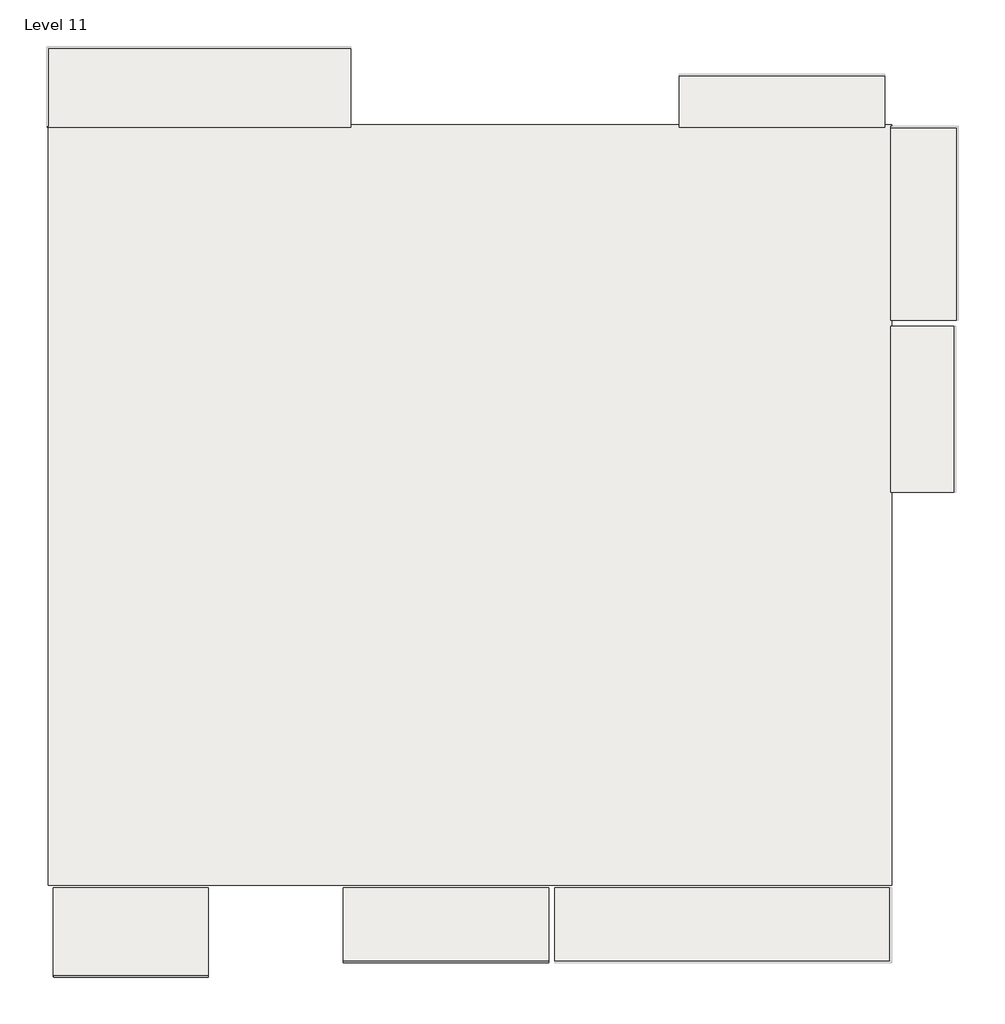
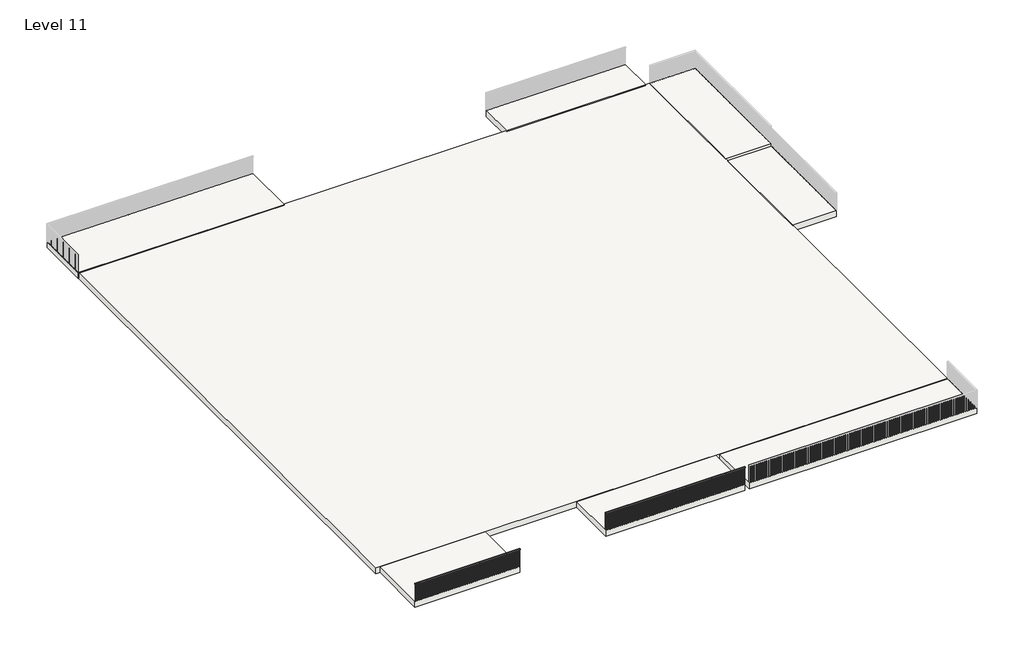
# One storey, part 1 of 5: 8 slabs, 2 railings.
"""IFC4 building model written with IfcOpenShell, lengths in millimetres."""

from ifc_helpers import new_model, si_unit, frame, origin, place, context, project, spatial, polyline, outline, extrude, element, save

model = new_model("IFC4")

# Units and contexts
model_context = context("Model", 3, world=origin())
ifc_project = project(units=[si_unit("LENGTHUNIT", "METRE", prefix="MILLI")], contexts=[model_context])

# Site, building, storey
site = spatial("IfcSite", under=ifc_project)
building = spatial("IfcBuilding", under=site)
storey = spatial("IfcBuildingStorey", under=building, Name="Level 11", Elevation=15544.8)

# Railings
placement = place(None, origin())
element("IfcRailing", 1, ObjectType="Handrail - Rectangular", at=placement, inside=storey, context=model_context, shape_type="SweptSolid", body=[
    extrude(outline(polyline([(-13617.5638778, -13399.9762475), (-13617.5638778, -13349.1762475), (-8499.4638778, -13349.1762475), (-8499.4638778, -13399.9762475), (-13617.5638778, -13399.9762475)])), frame((0.0, 0.0, 16408.4), z_axis=(0.0, 0.0, 1.0), x_axis=(1.0, 0.0, 0.0)), (0.0, 0.0, 1.0), 50.8),
    extrude(outline(polyline([(-8547.0888778, -13384.1012475), (-8547.0888778, -13365.0512475), (-8528.0388778, -13365.0512475), (-8528.0388778, -13384.1012475), (-8547.0888778, -13384.1012475)])), frame((0.0, 0.0, 15544.8), z_axis=(0.0, 0.0, 1.0), x_axis=(1.0, 0.0, 0.0)), (0.0, 0.0, 1.0), 863.6),
    extrude(outline(polyline([(-8648.6888778, -13384.1012475), (-8648.6888778, -13365.0512475), (-8629.6388778, -13365.0512475), (-8629.6388778, -13384.1012475), (-8648.6888778, -13384.1012475)])), frame((0.0, 0.0, 15544.8), z_axis=(0.0, 0.0, 1.0), x_axis=(1.0, 0.0, 0.0)), (0.0, 0.0, 1.0), 863.6),
    extrude(outline(polyline([(-8750.2888778, -13384.1012475), (-8750.2888778, -13365.0512475), (-8731.2388778, -13365.0512475), (-8731.2388778, -13384.1012475), (-8750.2888778, -13384.1012475)])), frame((0.0, 0.0, 15544.8), z_axis=(0.0, 0.0, 1.0), x_axis=(1.0, 0.0, 0.0)), (0.0, 0.0, 1.0), 863.6),
    extrude(outline(polyline([(-8851.8888778, -13384.1012475), (-8851.8888778, -13365.0512475), (-8832.8388778, -13365.0512475), (-8832.8388778, -13384.1012475), (-8851.8888778, -13384.1012475)])), frame((0.0, 0.0, 15544.8), z_axis=(0.0, 0.0, 1.0), x_axis=(1.0, 0.0, 0.0)), (0.0, 0.0, 1.0), 863.6),
    extrude(outline(polyline([(-8953.4888778, -13384.1012475), (-8953.4888778, -13365.0512475), (-8934.4388778, -13365.0512475), (-8934.4388778, -13384.1012475), (-8953.4888778, -13384.1012475)])), frame((0.0, 0.0, 15544.8), z_axis=(0.0, 0.0, 1.0), x_axis=(1.0, 0.0, 0.0)), (0.0, 0.0, 1.0), 863.6),
    extrude(outline(polyline([(-9055.0888778, -13384.1012475), (-9055.0888778, -13365.0512475), (-9036.0388778, -13365.0512475), (-9036.0388778, -13384.1012475), (-9055.0888778, -13384.1012475)])), frame((0.0, 0.0, 15544.8), z_axis=(0.0, 0.0, 1.0), x_axis=(1.0, 0.0, 0.0)), (0.0, 0.0, 1.0), 863.6),
    extrude(outline(polyline([(-9156.6888778, -13384.1012475), (-9156.6888778, -13365.0512475), (-9137.6388778, -13365.0512475), (-9137.6388778, -13384.1012475), (-9156.6888778, -13384.1012475)])), frame((0.0, 0.0, 15544.8), z_axis=(0.0, 0.0, 1.0), x_axis=(1.0, 0.0, 0.0)), (0.0, 0.0, 1.0), 863.6),
    extrude(outline(polyline([(-9258.2888778, -13384.1012475), (-9258.2888778, -13365.0512475), (-9239.2388778, -13365.0512475), (-9239.2388778, -13384.1012475), (-9258.2888778, -13384.1012475)])), frame((0.0, 0.0, 15544.8), z_axis=(0.0, 0.0, 1.0), x_axis=(1.0, 0.0, 0.0)), (0.0, 0.0, 1.0), 863.6),
    extrude(outline(polyline([(-9359.8888778, -13384.1012475), (-9359.8888778, -13365.0512475), (-9340.8388778, -13365.0512475), (-9340.8388778, -13384.1012475), (-9359.8888778, -13384.1012475)])), frame((0.0, 0.0, 15544.8), z_axis=(0.0, 0.0, 1.0), x_axis=(1.0, 0.0, 0.0)), (0.0, 0.0, 1.0), 863.6),
    extrude(outline(polyline([(-9461.4888778, -13384.1012475), (-9461.4888778, -13365.0512475), (-9442.4388778, -13365.0512475), (-9442.4388778, -13384.1012475), (-9461.4888778, -13384.1012475)])), frame((0.0, 0.0, 15544.8), z_axis=(0.0, 0.0, 1.0), x_axis=(1.0, 0.0, 0.0)), (0.0, 0.0, 1.0), 863.6),
    extrude(outline(polyline([(-9563.0888778, -13384.1012475), (-9563.0888778, -13365.0512475), (-9544.0388778, -13365.0512475), (-9544.0388778, -13384.1012475), (-9563.0888778, -13384.1012475)])), frame((0.0, 0.0, 15544.8), z_axis=(0.0, 0.0, 1.0), x_axis=(1.0, 0.0, 0.0)), (0.0, 0.0, 1.0), 863.6),
    extrude(outline(polyline([(-9664.6888778, -13384.1012475), (-9664.6888778, -13365.0512475), (-9645.6388778, -13365.0512475), (-9645.6388778, -13384.1012475), (-9664.6888778, -13384.1012475)])), frame((0.0, 0.0, 15544.8), z_axis=(0.0, 0.0, 1.0), x_axis=(1.0, 0.0, 0.0)), (0.0, 0.0, 1.0), 863.6),
    extrude(outline(polyline([(-9766.2888778, -13384.1012475), (-9766.2888778, -13365.0512475), (-9747.2388778, -13365.0512475), (-9747.2388778, -13384.1012475), (-9766.2888778, -13384.1012475)])), frame((0.0, 0.0, 15544.8), z_axis=(0.0, 0.0, 1.0), x_axis=(1.0, 0.0, 0.0)), (0.0, 0.0, 1.0), 863.6),
    extrude(outline(polyline([(-9867.8888778, -13384.1012475), (-9867.8888778, -13365.0512475), (-9848.8388778, -13365.0512475), (-9848.8388778, -13384.1012475), (-9867.8888778, -13384.1012475)])), frame((0.0, 0.0, 15544.8), z_axis=(0.0, 0.0, 1.0), x_axis=(1.0, 0.0, 0.0)), (0.0, 0.0, 1.0), 863.6),
    extrude(outline(polyline([(-9969.4888778, -13384.1012475), (-9969.4888778, -13365.0512475), (-9950.4388778, -13365.0512475), (-9950.4388778, -13384.1012475), (-9969.4888778, -13384.1012475)])), frame((0.0, 0.0, 15544.8), z_axis=(0.0, 0.0, 1.0), x_axis=(1.0, 0.0, 0.0)), (0.0, 0.0, 1.0), 863.6),
    extrude(outline(polyline([(-10071.0888778, -13384.1012475), (-10071.0888778, -13365.0512475), (-10052.0388778, -13365.0512475), (-10052.0388778, -13384.1012475), (-10071.0888778, -13384.1012475)])), frame((0.0, 0.0, 15544.8), z_axis=(0.0, 0.0, 1.0), x_axis=(1.0, 0.0, 0.0)), (0.0, 0.0, 1.0), 863.6),
    extrude(outline(polyline([(-10172.6888778, -13384.1012475), (-10172.6888778, -13365.0512475), (-10153.6388778, -13365.0512475), (-10153.6388778, -13384.1012475), (-10172.6888778, -13384.1012475)])), frame((0.0, 0.0, 15544.8), z_axis=(0.0, 0.0, 1.0), x_axis=(1.0, 0.0, 0.0)), (0.0, 0.0, 1.0), 863.6),
    extrude(outline(polyline([(-10274.2888778, -13384.1012475), (-10274.2888778, -13365.0512475), (-10255.2388778, -13365.0512475), (-10255.2388778, -13384.1012475), (-10274.2888778, -13384.1012475)])), frame((0.0, 0.0, 15544.8), z_axis=(0.0, 0.0, 1.0), x_axis=(1.0, 0.0, 0.0)), (0.0, 0.0, 1.0), 863.6),
    extrude(outline(polyline([(-10375.8888778, -13384.1012475), (-10375.8888778, -13365.0512475), (-10356.8388778, -13365.0512475), (-10356.8388778, -13384.1012475), (-10375.8888778, -13384.1012475)])), frame((0.0, 0.0, 15544.8), z_axis=(0.0, 0.0, 1.0), x_axis=(1.0, 0.0, 0.0)), (0.0, 0.0, 1.0), 863.6),
    extrude(outline(polyline([(-10477.4888778, -13384.1012475), (-10477.4888778, -13365.0512475), (-10458.4388778, -13365.0512475), (-10458.4388778, -13384.1012475), (-10477.4888778, -13384.1012475)])), frame((0.0, 0.0, 15544.8), z_axis=(0.0, 0.0, 1.0), x_axis=(1.0, 0.0, 0.0)), (0.0, 0.0, 1.0), 863.6),
    extrude(outline(polyline([(-10579.0888778, -13384.1012475), (-10579.0888778, -13365.0512475), (-10560.0388778, -13365.0512475), (-10560.0388778, -13384.1012475), (-10579.0888778, -13384.1012475)])), frame((0.0, 0.0, 15544.8), z_axis=(0.0, 0.0, 1.0), x_axis=(1.0, 0.0, 0.0)), (0.0, 0.0, 1.0), 863.6),
    extrude(outline(polyline([(-10680.6888778, -13384.1012475), (-10680.6888778, -13365.0512475), (-10661.6388778, -13365.0512475), (-10661.6388778, -13384.1012475), (-10680.6888778, -13384.1012475)])), frame((0.0, 0.0, 15544.8), z_axis=(0.0, 0.0, 1.0), x_axis=(1.0, 0.0, 0.0)), (0.0, 0.0, 1.0), 863.6),
    extrude(outline(polyline([(-10782.2888778, -13384.1012475), (-10782.2888778, -13365.0512475), (-10763.2388778, -13365.0512475), (-10763.2388778, -13384.1012475), (-10782.2888778, -13384.1012475)])), frame((0.0, 0.0, 15544.8), z_axis=(0.0, 0.0, 1.0), x_axis=(1.0, 0.0, 0.0)), (0.0, 0.0, 1.0), 863.6),
    extrude(outline(polyline([(-10883.8888778, -13384.1012475), (-10883.8888778, -13365.0512475), (-10864.8388778, -13365.0512475), (-10864.8388778, -13384.1012475), (-10883.8888778, -13384.1012475)])), frame((0.0, 0.0, 15544.8), z_axis=(0.0, 0.0, 1.0), x_axis=(1.0, 0.0, 0.0)), (0.0, 0.0, 1.0), 863.6),
    extrude(outline(polyline([(-10985.4888778, -13384.1012475), (-10985.4888778, -13365.0512475), (-10966.4388778, -13365.0512475), (-10966.4388778, -13384.1012475), (-10985.4888778, -13384.1012475)])), frame((0.0, 0.0, 15544.8), z_axis=(0.0, 0.0, 1.0), x_axis=(1.0, 0.0, 0.0)), (0.0, 0.0, 1.0), 863.6),
    extrude(outline(polyline([(-11087.0888778, -13384.1012475), (-11087.0888778, -13365.0512475), (-11068.0388778, -13365.0512475), (-11068.0388778, -13384.1012475), (-11087.0888778, -13384.1012475)])), frame((0.0, 0.0, 15544.8), z_axis=(0.0, 0.0, 1.0), x_axis=(1.0, 0.0, 0.0)), (0.0, 0.0, 1.0), 863.6),
    extrude(outline(polyline([(-11188.6888778, -13384.1012475), (-11188.6888778, -13365.0512475), (-11169.6388778, -13365.0512475), (-11169.6388778, -13384.1012475), (-11188.6888778, -13384.1012475)])), frame((0.0, 0.0, 15544.8), z_axis=(0.0, 0.0, 1.0), x_axis=(1.0, 0.0, 0.0)), (0.0, 0.0, 1.0), 863.6),
    extrude(outline(polyline([(-11290.2888778, -13384.1012475), (-11290.2888778, -13365.0512475), (-11271.2388778, -13365.0512475), (-11271.2388778, -13384.1012475), (-11290.2888778, -13384.1012475)])), frame((0.0, 0.0, 15544.8), z_axis=(0.0, 0.0, 1.0), x_axis=(1.0, 0.0, 0.0)), (0.0, 0.0, 1.0), 863.6),
    extrude(outline(polyline([(-11391.8888778, -13384.1012475), (-11391.8888778, -13365.0512475), (-11372.8388778, -13365.0512475), (-11372.8388778, -13384.1012475), (-11391.8888778, -13384.1012475)])), frame((0.0, 0.0, 15544.8), z_axis=(0.0, 0.0, 1.0), x_axis=(1.0, 0.0, 0.0)), (0.0, 0.0, 1.0), 863.6),
    extrude(outline(polyline([(-11493.4888778, -13384.1012475), (-11493.4888778, -13365.0512475), (-11474.4388778, -13365.0512475), (-11474.4388778, -13384.1012475), (-11493.4888778, -13384.1012475)])), frame((0.0, 0.0, 15544.8), z_axis=(0.0, 0.0, 1.0), x_axis=(1.0, 0.0, 0.0)), (0.0, 0.0, 1.0), 863.6),
    extrude(outline(polyline([(-11595.0888778, -13384.1012475), (-11595.0888778, -13365.0512475), (-11576.0388778, -13365.0512475), (-11576.0388778, -13384.1012475), (-11595.0888778, -13384.1012475)])), frame((0.0, 0.0, 15544.8), z_axis=(0.0, 0.0, 1.0), x_axis=(1.0, 0.0, 0.0)), (0.0, 0.0, 1.0), 863.6),
    extrude(outline(polyline([(-11696.6888778, -13384.1012475), (-11696.6888778, -13365.0512475), (-11677.6388778, -13365.0512475), (-11677.6388778, -13384.1012475), (-11696.6888778, -13384.1012475)])), frame((0.0, 0.0, 15544.8), z_axis=(0.0, 0.0, 1.0), x_axis=(1.0, 0.0, 0.0)), (0.0, 0.0, 1.0), 863.6),
    extrude(outline(polyline([(-11798.2888778, -13384.1012475), (-11798.2888778, -13365.0512475), (-11779.2388778, -13365.0512475), (-11779.2388778, -13384.1012475), (-11798.2888778, -13384.1012475)])), frame((0.0, 0.0, 15544.8), z_axis=(0.0, 0.0, 1.0), x_axis=(1.0, 0.0, 0.0)), (0.0, 0.0, 1.0), 863.6),
    extrude(outline(polyline([(-11899.8888778, -13384.1012475), (-11899.8888778, -13365.0512475), (-11880.8388778, -13365.0512475), (-11880.8388778, -13384.1012475), (-11899.8888778, -13384.1012475)])), frame((0.0, 0.0, 15544.8), z_axis=(0.0, 0.0, 1.0), x_axis=(1.0, 0.0, 0.0)), (0.0, 0.0, 1.0), 863.6),
    extrude(outline(polyline([(-12001.4888778, -13384.1012475), (-12001.4888778, -13365.0512475), (-11982.4388778, -13365.0512475), (-11982.4388778, -13384.1012475), (-12001.4888778, -13384.1012475)])), frame((0.0, 0.0, 15544.8), z_axis=(0.0, 0.0, 1.0), x_axis=(1.0, 0.0, 0.0)), (0.0, 0.0, 1.0), 863.6),
    extrude(outline(polyline([(-12103.0888778, -13384.1012475), (-12103.0888778, -13365.0512475), (-12084.0388778, -13365.0512475), (-12084.0388778, -13384.1012475), (-12103.0888778, -13384.1012475)])), frame((0.0, 0.0, 15544.8), z_axis=(0.0, 0.0, 1.0), x_axis=(1.0, 0.0, 0.0)), (0.0, 0.0, 1.0), 863.6),
    extrude(outline(polyline([(-12204.6888778, -13384.1012475), (-12204.6888778, -13365.0512475), (-12185.6388778, -13365.0512475), (-12185.6388778, -13384.1012475), (-12204.6888778, -13384.1012475)])), frame((0.0, 0.0, 15544.8), z_axis=(0.0, 0.0, 1.0), x_axis=(1.0, 0.0, 0.0)), (0.0, 0.0, 1.0), 863.6),
    extrude(outline(polyline([(-12306.2888778, -13384.1012475), (-12306.2888778, -13365.0512475), (-12287.2388778, -13365.0512475), (-12287.2388778, -13384.1012475), (-12306.2888778, -13384.1012475)])), frame((0.0, 0.0, 15544.8), z_axis=(0.0, 0.0, 1.0), x_axis=(1.0, 0.0, 0.0)), (0.0, 0.0, 1.0), 863.6),
    extrude(outline(polyline([(-12407.8888778, -13384.1012475), (-12407.8888778, -13365.0512475), (-12388.8388778, -13365.0512475), (-12388.8388778, -13384.1012475), (-12407.8888778, -13384.1012475)])), frame((0.0, 0.0, 15544.8), z_axis=(0.0, 0.0, 1.0), x_axis=(1.0, 0.0, 0.0)), (0.0, 0.0, 1.0), 863.6),
    extrude(outline(polyline([(-12509.4888778, -13384.1012475), (-12509.4888778, -13365.0512475), (-12490.4388778, -13365.0512475), (-12490.4388778, -13384.1012475), (-12509.4888778, -13384.1012475)])), frame((0.0, 0.0, 15544.8), z_axis=(0.0, 0.0, 1.0), x_axis=(1.0, 0.0, 0.0)), (0.0, 0.0, 1.0), 863.6),
    extrude(outline(polyline([(-12611.0888778, -13384.1012475), (-12611.0888778, -13365.0512475), (-12592.0388778, -13365.0512475), (-12592.0388778, -13384.1012475), (-12611.0888778, -13384.1012475)])), frame((0.0, 0.0, 15544.8), z_axis=(0.0, 0.0, 1.0), x_axis=(1.0, 0.0, 0.0)), (0.0, 0.0, 1.0), 863.6),
    extrude(outline(polyline([(-12712.6888778, -13384.1012475), (-12712.6888778, -13365.0512475), (-12693.6388778, -13365.0512475), (-12693.6388778, -13384.1012475), (-12712.6888778, -13384.1012475)])), frame((0.0, 0.0, 15544.8), z_axis=(0.0, 0.0, 1.0), x_axis=(1.0, 0.0, 0.0)), (0.0, 0.0, 1.0), 863.6),
    extrude(outline(polyline([(-12814.2888778, -13384.1012475), (-12814.2888778, -13365.0512475), (-12795.2388778, -13365.0512475), (-12795.2388778, -13384.1012475), (-12814.2888778, -13384.1012475)])), frame((0.0, 0.0, 15544.8), z_axis=(0.0, 0.0, 1.0), x_axis=(1.0, 0.0, 0.0)), (0.0, 0.0, 1.0), 863.6),
    extrude(outline(polyline([(-12915.8888778, -13384.1012475), (-12915.8888778, -13365.0512475), (-12896.8388778, -13365.0512475), (-12896.8388778, -13384.1012475), (-12915.8888778, -13384.1012475)])), frame((0.0, 0.0, 15544.8), z_axis=(0.0, 0.0, 1.0), x_axis=(1.0, 0.0, 0.0)), (0.0, 0.0, 1.0), 863.6),
    extrude(outline(polyline([(-13017.4888778, -13384.1012475), (-13017.4888778, -13365.0512475), (-12998.4388778, -13365.0512475), (-12998.4388778, -13384.1012475), (-13017.4888778, -13384.1012475)])), frame((0.0, 0.0, 15544.8), z_axis=(0.0, 0.0, 1.0), x_axis=(1.0, 0.0, 0.0)), (0.0, 0.0, 1.0), 863.6),
    extrude(outline(polyline([(-13119.0888778, -13384.1012475), (-13119.0888778, -13365.0512475), (-13100.0388778, -13365.0512475), (-13100.0388778, -13384.1012475), (-13119.0888778, -13384.1012475)])), frame((0.0, 0.0, 15544.8), z_axis=(0.0, 0.0, 1.0), x_axis=(1.0, 0.0, 0.0)), (0.0, 0.0, 1.0), 863.6),
    extrude(outline(polyline([(-13220.6888778, -13384.1012475), (-13220.6888778, -13365.0512475), (-13201.6388778, -13365.0512475), (-13201.6388778, -13384.1012475), (-13220.6888778, -13384.1012475)])), frame((0.0, 0.0, 15544.8), z_axis=(0.0, 0.0, 1.0), x_axis=(1.0, 0.0, 0.0)), (0.0, 0.0, 1.0), 863.6),
    extrude(outline(polyline([(-13322.2888778, -13384.1012475), (-13322.2888778, -13365.0512475), (-13303.2388778, -13365.0512475), (-13303.2388778, -13384.1012475), (-13322.2888778, -13384.1012475)])), frame((0.0, 0.0, 15544.8), z_axis=(0.0, 0.0, 1.0), x_axis=(1.0, 0.0, 0.0)), (0.0, 0.0, 1.0), 863.6),
    extrude(outline(polyline([(-13423.8888778, -13384.1012475), (-13423.8888778, -13365.0512475), (-13404.8388778, -13365.0512475), (-13404.8388778, -13384.1012475), (-13423.8888778, -13384.1012475)])), frame((0.0, 0.0, 15544.8), z_axis=(0.0, 0.0, 1.0), x_axis=(1.0, 0.0, 0.0)), (0.0, 0.0, 1.0), 863.6),
    extrude(outline(polyline([(-13525.4888778, -13384.1012475), (-13525.4888778, -13365.0512475), (-13506.4388778, -13365.0512475), (-13506.4388778, -13384.1012475), (-13525.4888778, -13384.1012475)])), frame((0.0, 0.0, 15544.8), z_axis=(0.0, 0.0, 1.0), x_axis=(1.0, 0.0, 0.0)), (0.0, 0.0, 1.0), 863.6),
    extrude(outline(polyline([(-8518.5138778, -13384.1012475), (-8518.5138778, -13365.0512475), (-8499.4638778, -13365.0512475), (-8499.4638778, -13384.1012475), (-8518.5138778, -13384.1012475)])), frame((0.0, 0.0, 15544.8), z_axis=(0.0, 0.0, 1.0), x_axis=(1.0, 0.0, 0.0)), (0.0, 0.0, 1.0), 863.6),
    extrude(outline(polyline([(-13617.5638778, -13384.1012475), (-13617.5638778, -13365.0512475), (-13598.5138778, -13365.0512475), (-13598.5138778, -13384.1012475), (-13617.5638778, -13384.1012475)])), frame((0.0, 0.0, 15544.8), z_axis=(0.0, 0.0, 1.0), x_axis=(1.0, 0.0, 0.0)), (0.0, 0.0, 1.0), 863.6),
])
element("IfcRailing", 2, ObjectType="Handrail - Rectangular", at=placement, inside=storey, context=model_context, shape_type="SweptSolid", body=[
    extrude(outline(polyline([(-4029.0638778, -12911.7749501), (-4029.0638778, -12860.9749501), (2778.1361222, -12860.9749501), (2778.1361222, -12911.7749501), (-4029.0638778, -12911.7749501)])), frame((0.0, 0.0, 16408.4), z_axis=(0.0, 0.0, 1.0), x_axis=(1.0, 0.0, 0.0)), (0.0, 0.0, 1.0), 50.8),
    extrude(outline(polyline([(2667.0111222, -12895.8999501), (2667.0111222, -12876.8499501), (2686.0611222, -12876.8499501), (2686.0611222, -12895.8999501), (2667.0111222, -12895.8999501)])), frame((0.0, 0.0, 15544.8), z_axis=(0.0, 0.0, 1.0), x_axis=(1.0, 0.0, 0.0)), (0.0, 0.0, 1.0), 863.6),
    extrude(outline(polyline([(2565.4111222, -12895.8999501), (2565.4111222, -12876.8499501), (2584.4611222, -12876.8499501), (2584.4611222, -12895.8999501), (2565.4111222, -12895.8999501)])), frame((0.0, 0.0, 15544.8), z_axis=(0.0, 0.0, 1.0), x_axis=(1.0, 0.0, 0.0)), (0.0, 0.0, 1.0), 863.6),
    extrude(outline(polyline([(2463.8111222, -12895.8999501), (2463.8111222, -12876.8499501), (2482.8611222, -12876.8499501), (2482.8611222, -12895.8999501), (2463.8111222, -12895.8999501)])), frame((0.0, 0.0, 15544.8), z_axis=(0.0, 0.0, 1.0), x_axis=(1.0, 0.0, 0.0)), (0.0, 0.0, 1.0), 863.6),
    extrude(outline(polyline([(2362.2111222, -12895.8999501), (2362.2111222, -12876.8499501), (2381.2611222, -12876.8499501), (2381.2611222, -12895.8999501), (2362.2111222, -12895.8999501)])), frame((0.0, 0.0, 15544.8), z_axis=(0.0, 0.0, 1.0), x_axis=(1.0, 0.0, 0.0)), (0.0, 0.0, 1.0), 863.6),
    extrude(outline(polyline([(2260.6111222, -12895.8999501), (2260.6111222, -12876.8499501), (2279.6611222, -12876.8499501), (2279.6611222, -12895.8999501), (2260.6111222, -12895.8999501)])), frame((0.0, 0.0, 15544.8), z_axis=(0.0, 0.0, 1.0), x_axis=(1.0, 0.0, 0.0)), (0.0, 0.0, 1.0), 863.6),
    extrude(outline(polyline([(2159.0111222, -12895.8999501), (2159.0111222, -12876.8499501), (2178.0611222, -12876.8499501), (2178.0611222, -12895.8999501), (2159.0111222, -12895.8999501)])), frame((0.0, 0.0, 15544.8), z_axis=(0.0, 0.0, 1.0), x_axis=(1.0, 0.0, 0.0)), (0.0, 0.0, 1.0), 863.6),
    extrude(outline(polyline([(2057.4111222, -12895.8999501), (2057.4111222, -12876.8499501), (2076.4611222, -12876.8499501), (2076.4611222, -12895.8999501), (2057.4111222, -12895.8999501)])), frame((0.0, 0.0, 15544.8), z_axis=(0.0, 0.0, 1.0), x_axis=(1.0, 0.0, 0.0)), (0.0, 0.0, 1.0), 863.6),
    extrude(outline(polyline([(1955.8111222, -12895.8999501), (1955.8111222, -12876.8499501), (1974.8611222, -12876.8499501), (1974.8611222, -12895.8999501), (1955.8111222, -12895.8999501)])), frame((0.0, 0.0, 15544.8), z_axis=(0.0, 0.0, 1.0), x_axis=(1.0, 0.0, 0.0)), (0.0, 0.0, 1.0), 863.6),
    extrude(outline(polyline([(1854.2111222, -12895.8999501), (1854.2111222, -12876.8499501), (1873.2611222, -12876.8499501), (1873.2611222, -12895.8999501), (1854.2111222, -12895.8999501)])), frame((0.0, 0.0, 15544.8), z_axis=(0.0, 0.0, 1.0), x_axis=(1.0, 0.0, 0.0)), (0.0, 0.0, 1.0), 863.6),
    extrude(outline(polyline([(1752.6111222, -12895.8999501), (1752.6111222, -12876.8499501), (1771.6611222, -12876.8499501), (1771.6611222, -12895.8999501), (1752.6111222, -12895.8999501)])), frame((0.0, 0.0, 15544.8), z_axis=(0.0, 0.0, 1.0), x_axis=(1.0, 0.0, 0.0)), (0.0, 0.0, 1.0), 863.6),
    extrude(outline(polyline([(1651.0111222, -12895.8999501), (1651.0111222, -12876.8499501), (1670.0611222, -12876.8499501), (1670.0611222, -12895.8999501), (1651.0111222, -12895.8999501)])), frame((0.0, 0.0, 15544.8), z_axis=(0.0, 0.0, 1.0), x_axis=(1.0, 0.0, 0.0)), (0.0, 0.0, 1.0), 863.6),
    extrude(outline(polyline([(1549.4111222, -12895.8999501), (1549.4111222, -12876.8499501), (1568.4611222, -12876.8499501), (1568.4611222, -12895.8999501), (1549.4111222, -12895.8999501)])), frame((0.0, 0.0, 15544.8), z_axis=(0.0, 0.0, 1.0), x_axis=(1.0, 0.0, 0.0)), (0.0, 0.0, 1.0), 863.6),
    extrude(outline(polyline([(1447.8111222, -12895.8999501), (1447.8111222, -12876.8499501), (1466.8611222, -12876.8499501), (1466.8611222, -12895.8999501), (1447.8111222, -12895.8999501)])), frame((0.0, 0.0, 15544.8), z_axis=(0.0, 0.0, 1.0), x_axis=(1.0, 0.0, 0.0)), (0.0, 0.0, 1.0), 863.6),
    extrude(outline(polyline([(1346.2111222, -12895.8999501), (1346.2111222, -12876.8499501), (1365.2611222, -12876.8499501), (1365.2611222, -12895.8999501), (1346.2111222, -12895.8999501)])), frame((0.0, 0.0, 15544.8), z_axis=(0.0, 0.0, 1.0), x_axis=(1.0, 0.0, 0.0)), (0.0, 0.0, 1.0), 863.6),
    extrude(outline(polyline([(1244.6111222, -12895.8999501), (1244.6111222, -12876.8499501), (1263.6611222, -12876.8499501), (1263.6611222, -12895.8999501), (1244.6111222, -12895.8999501)])), frame((0.0, 0.0, 15544.8), z_axis=(0.0, 0.0, 1.0), x_axis=(1.0, 0.0, 0.0)), (0.0, 0.0, 1.0), 863.6),
    extrude(outline(polyline([(1143.0111222, -12895.8999501), (1143.0111222, -12876.8499501), (1162.0611222, -12876.8499501), (1162.0611222, -12895.8999501), (1143.0111222, -12895.8999501)])), frame((0.0, 0.0, 15544.8), z_axis=(0.0, 0.0, 1.0), x_axis=(1.0, 0.0, 0.0)), (0.0, 0.0, 1.0), 863.6),
    extrude(outline(polyline([(1041.4111222, -12895.8999501), (1041.4111222, -12876.8499501), (1060.4611222, -12876.8499501), (1060.4611222, -12895.8999501), (1041.4111222, -12895.8999501)])), frame((0.0, 0.0, 15544.8), z_axis=(0.0, 0.0, 1.0), x_axis=(1.0, 0.0, 0.0)), (0.0, 0.0, 1.0), 863.6),
    extrude(outline(polyline([(939.8111222, -12895.8999501), (939.8111222, -12876.8499501), (958.8611222, -12876.8499501), (958.8611222, -12895.8999501), (939.8111222, -12895.8999501)])), frame((0.0, 0.0, 15544.8), z_axis=(0.0, 0.0, 1.0), x_axis=(1.0, 0.0, 0.0)), (0.0, 0.0, 1.0), 863.6),
    extrude(outline(polyline([(838.2111222, -12895.8999501), (838.2111222, -12876.8499501), (857.2611222, -12876.8499501), (857.2611222, -12895.8999501), (838.2111222, -12895.8999501)])), frame((0.0, 0.0, 15544.8), z_axis=(0.0, 0.0, 1.0), x_axis=(1.0, 0.0, 0.0)), (0.0, 0.0, 1.0), 863.6),
    extrude(outline(polyline([(736.6111222, -12895.8999501), (736.6111222, -12876.8499501), (755.6611222, -12876.8499501), (755.6611222, -12895.8999501), (736.6111222, -12895.8999501)])), frame((0.0, 0.0, 15544.8), z_axis=(0.0, 0.0, 1.0), x_axis=(1.0, 0.0, 0.0)), (0.0, 0.0, 1.0), 863.6),
    extrude(outline(polyline([(635.0111222, -12895.8999501), (635.0111222, -12876.8499501), (654.0611222, -12876.8499501), (654.0611222, -12895.8999501), (635.0111222, -12895.8999501)])), frame((0.0, 0.0, 15544.8), z_axis=(0.0, 0.0, 1.0), x_axis=(1.0, 0.0, 0.0)), (0.0, 0.0, 1.0), 863.6),
    extrude(outline(polyline([(533.4111222, -12895.8999501), (533.4111222, -12876.8499501), (552.4611222, -12876.8499501), (552.4611222, -12895.8999501), (533.4111222, -12895.8999501)])), frame((0.0, 0.0, 15544.8), z_axis=(0.0, 0.0, 1.0), x_axis=(1.0, 0.0, 0.0)), (0.0, 0.0, 1.0), 863.6),
    extrude(outline(polyline([(431.8111222, -12895.8999501), (431.8111222, -12876.8499501), (450.8611222, -12876.8499501), (450.8611222, -12895.8999501), (431.8111222, -12895.8999501)])), frame((0.0, 0.0, 15544.8), z_axis=(0.0, 0.0, 1.0), x_axis=(1.0, 0.0, 0.0)), (0.0, 0.0, 1.0), 863.6),
    extrude(outline(polyline([(330.2111222, -12895.8999501), (330.2111222, -12876.8499501), (349.2611222, -12876.8499501), (349.2611222, -12895.8999501), (330.2111222, -12895.8999501)])), frame((0.0, 0.0, 15544.8), z_axis=(0.0, 0.0, 1.0), x_axis=(1.0, 0.0, 0.0)), (0.0, 0.0, 1.0), 863.6),
    extrude(outline(polyline([(228.6111222, -12895.8999501), (228.6111222, -12876.8499501), (247.6611222, -12876.8499501), (247.6611222, -12895.8999501), (228.6111222, -12895.8999501)])), frame((0.0, 0.0, 15544.8), z_axis=(0.0, 0.0, 1.0), x_axis=(1.0, 0.0, 0.0)), (0.0, 0.0, 1.0), 863.6),
    extrude(outline(polyline([(127.0111222, -12895.8999501), (127.0111222, -12876.8499501), (146.0611222, -12876.8499501), (146.0611222, -12895.8999501), (127.0111222, -12895.8999501)])), frame((0.0, 0.0, 15544.8), z_axis=(0.0, 0.0, 1.0), x_axis=(1.0, 0.0, 0.0)), (0.0, 0.0, 1.0), 863.6),
    extrude(outline(polyline([(25.4111222, -12895.8999501), (25.4111222, -12876.8499501), (44.4611222, -12876.8499501), (44.4611222, -12895.8999501), (25.4111222, -12895.8999501)])), frame((0.0, 0.0, 15544.8), z_axis=(0.0, 0.0, 1.0), x_axis=(1.0, 0.0, 0.0)), (0.0, 0.0, 1.0), 863.6),
    extrude(outline(polyline([(-76.1888778, -12895.8999501), (-76.1888778, -12876.8499501), (-57.1388778, -12876.8499501), (-57.1388778, -12895.8999501), (-76.1888778, -12895.8999501)])), frame((0.0, 0.0, 15544.8), z_axis=(0.0, 0.0, 1.0), x_axis=(1.0, 0.0, 0.0)), (0.0, 0.0, 1.0), 863.6),
    extrude(outline(polyline([(-177.7888778, -12895.8999501), (-177.7888778, -12876.8499501), (-158.7388778, -12876.8499501), (-158.7388778, -12895.8999501), (-177.7888778, -12895.8999501)])), frame((0.0, 0.0, 15544.8), z_axis=(0.0, 0.0, 1.0), x_axis=(1.0, 0.0, 0.0)), (0.0, 0.0, 1.0), 863.6),
    extrude(outline(polyline([(-279.3888778, -12895.8999501), (-279.3888778, -12876.8499501), (-260.3388778, -12876.8499501), (-260.3388778, -12895.8999501), (-279.3888778, -12895.8999501)])), frame((0.0, 0.0, 15544.8), z_axis=(0.0, 0.0, 1.0), x_axis=(1.0, 0.0, 0.0)), (0.0, 0.0, 1.0), 863.6),
    extrude(outline(polyline([(-380.9888778, -12895.8999501), (-380.9888778, -12876.8499501), (-361.9388778, -12876.8499501), (-361.9388778, -12895.8999501), (-380.9888778, -12895.8999501)])), frame((0.0, 0.0, 15544.8), z_axis=(0.0, 0.0, 1.0), x_axis=(1.0, 0.0, 0.0)), (0.0, 0.0, 1.0), 863.6),
    extrude(outline(polyline([(-482.5888778, -12895.8999501), (-482.5888778, -12876.8499501), (-463.5388778, -12876.8499501), (-463.5388778, -12895.8999501), (-482.5888778, -12895.8999501)])), frame((0.0, 0.0, 15544.8), z_axis=(0.0, 0.0, 1.0), x_axis=(1.0, 0.0, 0.0)), (0.0, 0.0, 1.0), 863.6),
    extrude(outline(polyline([(-584.1888778, -12895.8999501), (-584.1888778, -12876.8499501), (-565.1388778, -12876.8499501), (-565.1388778, -12895.8999501), (-584.1888778, -12895.8999501)])), frame((0.0, 0.0, 15544.8), z_axis=(0.0, 0.0, 1.0), x_axis=(1.0, 0.0, 0.0)), (0.0, 0.0, 1.0), 863.6),
    extrude(outline(polyline([(-685.7888778, -12895.8999501), (-685.7888778, -12876.8499501), (-666.7388778, -12876.8499501), (-666.7388778, -12895.8999501), (-685.7888778, -12895.8999501)])), frame((0.0, 0.0, 15544.8), z_axis=(0.0, 0.0, 1.0), x_axis=(1.0, 0.0, 0.0)), (0.0, 0.0, 1.0), 863.6),
    extrude(outline(polyline([(-787.3888778, -12895.8999501), (-787.3888778, -12876.8499501), (-768.3388778, -12876.8499501), (-768.3388778, -12895.8999501), (-787.3888778, -12895.8999501)])), frame((0.0, 0.0, 15544.8), z_axis=(0.0, 0.0, 1.0), x_axis=(1.0, 0.0, 0.0)), (0.0, 0.0, 1.0), 863.6),
    extrude(outline(polyline([(-888.9888778, -12895.8999501), (-888.9888778, -12876.8499501), (-869.9388778, -12876.8499501), (-869.9388778, -12895.8999501), (-888.9888778, -12895.8999501)])), frame((0.0, 0.0, 15544.8), z_axis=(0.0, 0.0, 1.0), x_axis=(1.0, 0.0, 0.0)), (0.0, 0.0, 1.0), 863.6),
    extrude(outline(polyline([(-990.5888778, -12895.8999501), (-990.5888778, -12876.8499501), (-971.5388778, -12876.8499501), (-971.5388778, -12895.8999501), (-990.5888778, -12895.8999501)])), frame((0.0, 0.0, 15544.8), z_axis=(0.0, 0.0, 1.0), x_axis=(1.0, 0.0, 0.0)), (0.0, 0.0, 1.0), 863.6),
    extrude(outline(polyline([(-1092.1888778, -12895.8999501), (-1092.1888778, -12876.8499501), (-1073.1388778, -12876.8499501), (-1073.1388778, -12895.8999501), (-1092.1888778, -12895.8999501)])), frame((0.0, 0.0, 15544.8), z_axis=(0.0, 0.0, 1.0), x_axis=(1.0, 0.0, 0.0)), (0.0, 0.0, 1.0), 863.6),
    extrude(outline(polyline([(-1193.7888778, -12895.8999501), (-1193.7888778, -12876.8499501), (-1174.7388778, -12876.8499501), (-1174.7388778, -12895.8999501), (-1193.7888778, -12895.8999501)])), frame((0.0, 0.0, 15544.8), z_axis=(0.0, 0.0, 1.0), x_axis=(1.0, 0.0, 0.0)), (0.0, 0.0, 1.0), 863.6),
    extrude(outline(polyline([(-1295.3888778, -12895.8999501), (-1295.3888778, -12876.8499501), (-1276.3388778, -12876.8499501), (-1276.3388778, -12895.8999501), (-1295.3888778, -12895.8999501)])), frame((0.0, 0.0, 15544.8), z_axis=(0.0, 0.0, 1.0), x_axis=(1.0, 0.0, 0.0)), (0.0, 0.0, 1.0), 863.6),
    extrude(outline(polyline([(-1396.9888778, -12895.8999501), (-1396.9888778, -12876.8499501), (-1377.9388778, -12876.8499501), (-1377.9388778, -12895.8999501), (-1396.9888778, -12895.8999501)])), frame((0.0, 0.0, 15544.8), z_axis=(0.0, 0.0, 1.0), x_axis=(1.0, 0.0, 0.0)), (0.0, 0.0, 1.0), 863.6),
    extrude(outline(polyline([(-1498.5888778, -12895.8999501), (-1498.5888778, -12876.8499501), (-1479.5388778, -12876.8499501), (-1479.5388778, -12895.8999501), (-1498.5888778, -12895.8999501)])), frame((0.0, 0.0, 15544.8), z_axis=(0.0, 0.0, 1.0), x_axis=(1.0, 0.0, 0.0)), (0.0, 0.0, 1.0), 863.6),
    extrude(outline(polyline([(-1600.1888778, -12895.8999501), (-1600.1888778, -12876.8499501), (-1581.1388778, -12876.8499501), (-1581.1388778, -12895.8999501), (-1600.1888778, -12895.8999501)])), frame((0.0, 0.0, 15544.8), z_axis=(0.0, 0.0, 1.0), x_axis=(1.0, 0.0, 0.0)), (0.0, 0.0, 1.0), 863.6),
    extrude(outline(polyline([(-1701.7888778, -12895.8999501), (-1701.7888778, -12876.8499501), (-1682.7388778, -12876.8499501), (-1682.7388778, -12895.8999501), (-1701.7888778, -12895.8999501)])), frame((0.0, 0.0, 15544.8), z_axis=(0.0, 0.0, 1.0), x_axis=(1.0, 0.0, 0.0)), (0.0, 0.0, 1.0), 863.6),
    extrude(outline(polyline([(-1803.3888778, -12895.8999501), (-1803.3888778, -12876.8499501), (-1784.3388778, -12876.8499501), (-1784.3388778, -12895.8999501), (-1803.3888778, -12895.8999501)])), frame((0.0, 0.0, 15544.8), z_axis=(0.0, 0.0, 1.0), x_axis=(1.0, 0.0, 0.0)), (0.0, 0.0, 1.0), 863.6),
    extrude(outline(polyline([(-1904.9888778, -12895.8999501), (-1904.9888778, -12876.8499501), (-1885.9388778, -12876.8499501), (-1885.9388778, -12895.8999501), (-1904.9888778, -12895.8999501)])), frame((0.0, 0.0, 15544.8), z_axis=(0.0, 0.0, 1.0), x_axis=(1.0, 0.0, 0.0)), (0.0, 0.0, 1.0), 863.6),
    extrude(outline(polyline([(-2006.5888778, -12895.8999501), (-2006.5888778, -12876.8499501), (-1987.5388778, -12876.8499501), (-1987.5388778, -12895.8999501), (-2006.5888778, -12895.8999501)])), frame((0.0, 0.0, 15544.8), z_axis=(0.0, 0.0, 1.0), x_axis=(1.0, 0.0, 0.0)), (0.0, 0.0, 1.0), 863.6),
    extrude(outline(polyline([(-2108.1888778, -12895.8999501), (-2108.1888778, -12876.8499501), (-2089.1388778, -12876.8499501), (-2089.1388778, -12895.8999501), (-2108.1888778, -12895.8999501)])), frame((0.0, 0.0, 15544.8), z_axis=(0.0, 0.0, 1.0), x_axis=(1.0, 0.0, 0.0)), (0.0, 0.0, 1.0), 863.6),
    extrude(outline(polyline([(-2209.7888778, -12895.8999501), (-2209.7888778, -12876.8499501), (-2190.7388778, -12876.8499501), (-2190.7388778, -12895.8999501), (-2209.7888778, -12895.8999501)])), frame((0.0, 0.0, 15544.8), z_axis=(0.0, 0.0, 1.0), x_axis=(1.0, 0.0, 0.0)), (0.0, 0.0, 1.0), 863.6),
    extrude(outline(polyline([(-2311.3888778, -12895.8999501), (-2311.3888778, -12876.8499501), (-2292.3388778, -12876.8499501), (-2292.3388778, -12895.8999501), (-2311.3888778, -12895.8999501)])), frame((0.0, 0.0, 15544.8), z_axis=(0.0, 0.0, 1.0), x_axis=(1.0, 0.0, 0.0)), (0.0, 0.0, 1.0), 863.6),
    extrude(outline(polyline([(-2412.9888778, -12895.8999501), (-2412.9888778, -12876.8499501), (-2393.9388778, -12876.8499501), (-2393.9388778, -12895.8999501), (-2412.9888778, -12895.8999501)])), frame((0.0, 0.0, 15544.8), z_axis=(0.0, 0.0, 1.0), x_axis=(1.0, 0.0, 0.0)), (0.0, 0.0, 1.0), 863.6),
    extrude(outline(polyline([(-2514.5888778, -12895.8999501), (-2514.5888778, -12876.8499501), (-2495.5388778, -12876.8499501), (-2495.5388778, -12895.8999501), (-2514.5888778, -12895.8999501)])), frame((0.0, 0.0, 15544.8), z_axis=(0.0, 0.0, 1.0), x_axis=(1.0, 0.0, 0.0)), (0.0, 0.0, 1.0), 863.6),
    extrude(outline(polyline([(-2616.1888778, -12895.8999501), (-2616.1888778, -12876.8499501), (-2597.1388778, -12876.8499501), (-2597.1388778, -12895.8999501), (-2616.1888778, -12895.8999501)])), frame((0.0, 0.0, 15544.8), z_axis=(0.0, 0.0, 1.0), x_axis=(1.0, 0.0, 0.0)), (0.0, 0.0, 1.0), 863.6),
    extrude(outline(polyline([(-2717.7888778, -12895.8999501), (-2717.7888778, -12876.8499501), (-2698.7388778, -12876.8499501), (-2698.7388778, -12895.8999501), (-2717.7888778, -12895.8999501)])), frame((0.0, 0.0, 15544.8), z_axis=(0.0, 0.0, 1.0), x_axis=(1.0, 0.0, 0.0)), (0.0, 0.0, 1.0), 863.6),
    extrude(outline(polyline([(-2819.3888778, -12895.8999501), (-2819.3888778, -12876.8499501), (-2800.3388778, -12876.8499501), (-2800.3388778, -12895.8999501), (-2819.3888778, -12895.8999501)])), frame((0.0, 0.0, 15544.8), z_axis=(0.0, 0.0, 1.0), x_axis=(1.0, 0.0, 0.0)), (0.0, 0.0, 1.0), 863.6),
    extrude(outline(polyline([(-2920.9888778, -12895.8999501), (-2920.9888778, -12876.8499501), (-2901.9388778, -12876.8499501), (-2901.9388778, -12895.8999501), (-2920.9888778, -12895.8999501)])), frame((0.0, 0.0, 15544.8), z_axis=(0.0, 0.0, 1.0), x_axis=(1.0, 0.0, 0.0)), (0.0, 0.0, 1.0), 863.6),
    extrude(outline(polyline([(-3022.5888778, -12895.8999501), (-3022.5888778, -12876.8499501), (-3003.5388778, -12876.8499501), (-3003.5388778, -12895.8999501), (-3022.5888778, -12895.8999501)])), frame((0.0, 0.0, 15544.8), z_axis=(0.0, 0.0, 1.0), x_axis=(1.0, 0.0, 0.0)), (0.0, 0.0, 1.0), 863.6),
    extrude(outline(polyline([(-3124.1888778, -12895.8999501), (-3124.1888778, -12876.8499501), (-3105.1388778, -12876.8499501), (-3105.1388778, -12895.8999501), (-3124.1888778, -12895.8999501)])), frame((0.0, 0.0, 15544.8), z_axis=(0.0, 0.0, 1.0), x_axis=(1.0, 0.0, 0.0)), (0.0, 0.0, 1.0), 863.6),
    extrude(outline(polyline([(-3225.7888778, -12895.8999501), (-3225.7888778, -12876.8499501), (-3206.7388778, -12876.8499501), (-3206.7388778, -12895.8999501), (-3225.7888778, -12895.8999501)])), frame((0.0, 0.0, 15544.8), z_axis=(0.0, 0.0, 1.0), x_axis=(1.0, 0.0, 0.0)), (0.0, 0.0, 1.0), 863.6),
    extrude(outline(polyline([(-3327.3888778, -12895.8999501), (-3327.3888778, -12876.8499501), (-3308.3388778, -12876.8499501), (-3308.3388778, -12895.8999501), (-3327.3888778, -12895.8999501)])), frame((0.0, 0.0, 15544.8), z_axis=(0.0, 0.0, 1.0), x_axis=(1.0, 0.0, 0.0)), (0.0, 0.0, 1.0), 863.6),
    extrude(outline(polyline([(-3428.9888778, -12895.8999501), (-3428.9888778, -12876.8499501), (-3409.9388778, -12876.8499501), (-3409.9388778, -12895.8999501), (-3428.9888778, -12895.8999501)])), frame((0.0, 0.0, 15544.8), z_axis=(0.0, 0.0, 1.0), x_axis=(1.0, 0.0, 0.0)), (0.0, 0.0, 1.0), 863.6),
    extrude(outline(polyline([(-3530.5888778, -12895.8999501), (-3530.5888778, -12876.8499501), (-3511.5388778, -12876.8499501), (-3511.5388778, -12895.8999501), (-3530.5888778, -12895.8999501)])), frame((0.0, 0.0, 15544.8), z_axis=(0.0, 0.0, 1.0), x_axis=(1.0, 0.0, 0.0)), (0.0, 0.0, 1.0), 863.6),
    extrude(outline(polyline([(-3632.1888778, -12895.8999501), (-3632.1888778, -12876.8499501), (-3613.1388778, -12876.8499501), (-3613.1388778, -12895.8999501), (-3632.1888778, -12895.8999501)])), frame((0.0, 0.0, 15544.8), z_axis=(0.0, 0.0, 1.0), x_axis=(1.0, 0.0, 0.0)), (0.0, 0.0, 1.0), 863.6),
    extrude(outline(polyline([(-3733.7888778, -12895.8999501), (-3733.7888778, -12876.8499501), (-3714.7388778, -12876.8499501), (-3714.7388778, -12895.8999501), (-3733.7888778, -12895.8999501)])), frame((0.0, 0.0, 15544.8), z_axis=(0.0, 0.0, 1.0), x_axis=(1.0, 0.0, 0.0)), (0.0, 0.0, 1.0), 863.6),
    extrude(outline(polyline([(-3835.3888778, -12895.8999501), (-3835.3888778, -12876.8499501), (-3816.3388778, -12876.8499501), (-3816.3388778, -12895.8999501), (-3835.3888778, -12895.8999501)])), frame((0.0, 0.0, 15544.8), z_axis=(0.0, 0.0, 1.0), x_axis=(1.0, 0.0, 0.0)), (0.0, 0.0, 1.0), 863.6),
    extrude(outline(polyline([(-3936.9888778, -12895.8999501), (-3936.9888778, -12876.8499501), (-3917.9388778, -12876.8499501), (-3917.9388778, -12895.8999501), (-3936.9888778, -12895.8999501)])), frame((0.0, 0.0, 15544.8), z_axis=(0.0, 0.0, 1.0), x_axis=(1.0, 0.0, 0.0)), (0.0, 0.0, 1.0), 863.6),
    extrude(outline(polyline([(2759.0861222, -12895.8999501), (2759.0861222, -12876.8499501), (2778.1361222, -12876.8499501), (2778.1361222, -12895.8999501), (2759.0861222, -12895.8999501)])), frame((0.0, 0.0, 15544.8), z_axis=(0.0, 0.0, 1.0), x_axis=(1.0, 0.0, 0.0)), (0.0, 0.0, 1.0), 863.6),
    extrude(outline(polyline([(-4029.0638778, -12895.8999501), (-4029.0638778, -12876.8499501), (-4010.0138778, -12876.8499501), (-4010.0138778, -12895.8999501), (-4029.0638778, -12895.8999501)])), frame((0.0, 0.0, 15544.8), z_axis=(0.0, 0.0, 1.0), x_axis=(1.0, 0.0, 0.0)), (0.0, 0.0, 1.0), 863.6),
])

# Slabs
element("IfcSlab", 3, at=placement, inside=storey, context=model_context, shape_type="SweptSolid", body=[
    extrude(outline(polyline([(14106.5361222, -10428.1762475), (14106.5361222, -12886.3749501), (2981.3361222, -12886.3749501), (2981.3361222, -10428.1762475), (14106.5361222, -10428.1762475)])), frame((0.0, 0.0, 15240.0), z_axis=(0.0, 0.0, 1.0), x_axis=(1.0, 0.0, 0.0)), (0.0, 0.0, 1.0), 304.8),
])
element("IfcSlab", 4, at=placement, inside=storey, context=model_context, shape_type="SweptSolid", body=[
    extrude(outline(polyline([(-8499.4638778, -10428.1762475), (-8499.4638778, -13374.5762475), (-13630.2638778, -13374.5762475), (-13630.2638778, -10428.1762475), (-8499.4638778, -10428.1762475)])), frame((0.0, 0.0, 15240.0), z_axis=(0.0, 0.0, 1.0), x_axis=(1.0, 0.0, 0.0)), (0.0, 0.0, 1.0), 304.8),
])
element("IfcSlab", 5, at=placement, inside=storey, context=model_context, shape_type="SweptSolid", body=[
    extrude(outline(polyline([(2778.1361222, -10428.1762475), (2778.1361222, -12886.3749501), (-4029.0638778, -12886.3749501), (-4029.0638778, -10428.1762475), (2778.1361222, -10428.1762475)])), frame((0.0, 0.0, 15240.0), z_axis=(0.0, 0.0, 1.0), x_axis=(1.0, 0.0, 0.0)), (0.0, 0.0, 1.0), 304.8),
])
element("IfcSlab", 6, at=placement, inside=storey, context=model_context, shape_type="SweptSolid", body=[
    extrude(outline(polyline([(16240.1361222, 8164.6237525), (16240.1361222, 2678.2237525), (14106.5361222, 2678.2237525), (14106.5361222, 8164.6237525), (16240.1361222, 8164.6237525)])), frame((0.0, 0.0, 15240.0), z_axis=(0.0, 0.0, 1.0), x_axis=(1.0, 0.0, 0.0)), (0.0, 0.0, 1.0), 304.8),
])
element("IfcSlab", 7, at=placement, inside=storey, context=model_context, shape_type="SweptSolid", body=[
    extrude(outline(polyline([(16321.4289933, 14768.6237525), (16321.4289933, 8367.8237525), (14106.5361222, 8367.8237525), (14106.5361222, 14768.6237525), (16321.4289933, 14768.6237525)])), frame((0.0, 0.0, 15240.0), z_axis=(0.0, 0.0, 1.0), x_axis=(1.0, 0.0, 0.0)), (0.0, 0.0, 1.0), 304.8),
])
element("IfcSlab", 8, at=placement, inside=storey, context=model_context, shape_type="SweptSolid", body=[
    extrude(outline(polyline([(13903.3361222, 14768.6237525), (7096.1361222, 14768.6237525), (7096.1361222, 16495.8237525), (13903.3361222, 16495.8237525), (13903.3361222, 14768.6237525)])), frame((0.0, 0.0, 15240.0), z_axis=(0.0, 0.0, 1.0), x_axis=(1.0, 0.0, 0.0)), (0.0, 0.0, 1.0), 304.8),
])
element("IfcSlab", 9, at=placement, inside=storey, context=model_context, shape_type="SweptSolid", body=[
    extrude(outline(polyline([(-13833.4638778, 14768.6237525), (-13833.4638778, 17410.2237525), (-3775.0638778, 17410.2237525), (-3775.0638778, 14768.6237525), (-13833.4638778, 14768.6237525)])), frame((0.0, 0.0, 15240.0), z_axis=(0.0, 0.0, 1.0), x_axis=(1.0, 0.0, 0.0)), (0.0, 0.0, 1.0), 304.8),
])
element("IfcSlab", 10, ObjectType="Generic - 12\"", at=placement, inside=storey, context=model_context, shape_type="SweptSolid", body=[
    extrude(outline(polyline([(14144.6361222, 14848.944107), (14144.6361222, -10347.855893), (-13795.3638778, -10347.855893), (-13795.3638778, 14848.944107), (14144.6361222, 14848.944107)])), frame((0.0, 0.0, 15193.6940312), z_axis=(0.0, 0.0, 1.0), x_axis=(1.0, 0.0, 0.0)), (0.0, 0.0, 1.0), 304.8),
])

save(model, "model.ifc")

# Revit data of these elements
# Type "Handrail - Rectangular"
#   Assembly Code = "C2010400"
#   built-in parameter 1008612 = 0.0416667 (stored number, unit not read)
#   built-in parameter 1008611 = 0.0416667 (stored number, unit not read)
#   built-in parameter 1008609 = 0.333333 (stored number, unit not read)
#   built-in parameter 1008604 = 0.166667 (stored number, unit not read)
#   built-in parameter 1008603 = 0.166667 (stored number, unit not read)
#   Railing Height = 3' - 0"
#   built-in parameter 1008630 = 2
#   built-in parameter 1008610 = 2
#   built-in parameter 1008618 = Baluster - Square : 3/4"
# Type
#   Assembly Code = "B1010"
#   Function = 0
#   Layers, outside or top first: 1' - 0" "Tile, Porcelain, 4in" (function 1)
# Type "Generic - 12\""
#   Assembly Code = "B1010"
#   Function = 0
#   Layers, outside or top first: 1' - 0" no material (function 1)
# Elements 1, 2 (IfcRailing, "Handrail - Rectangular")
#   Phase Created = New Construction
# Elements 3, 4, 5, 6, 7, 8 (IfcSlab)
#   Height Offset From Level = 0' - 0"
#   Phase Created = New Construction
#   Materials on its faces: "Tile, Porcelain, 4in"
# Element 9 (IfcSlab)
#   built-in parameter 1001955 = 3.14159 (stored number, unit not read)
#   Height Offset From Level = 0' - 0"
#   Phase Created = New Construction
#   Materials on its faces: "Tile, Porcelain, 4in"
# Element 10 (IfcSlab, "Generic - 12\"")
#   Height Offset From Level = -0' - 1.82307"
#   Phase Created = New Construction
#   Materials on its faces: "Default Floor"
# Materials
#   "Tile, Porcelain, 4in": class "Generic", colour RGB 89 87 158, transparency 0, Description = "Porcelain tile, 4\", white", Cost = 0
#   "Default Floor": colour RGB 128 128 128, transparency 0
